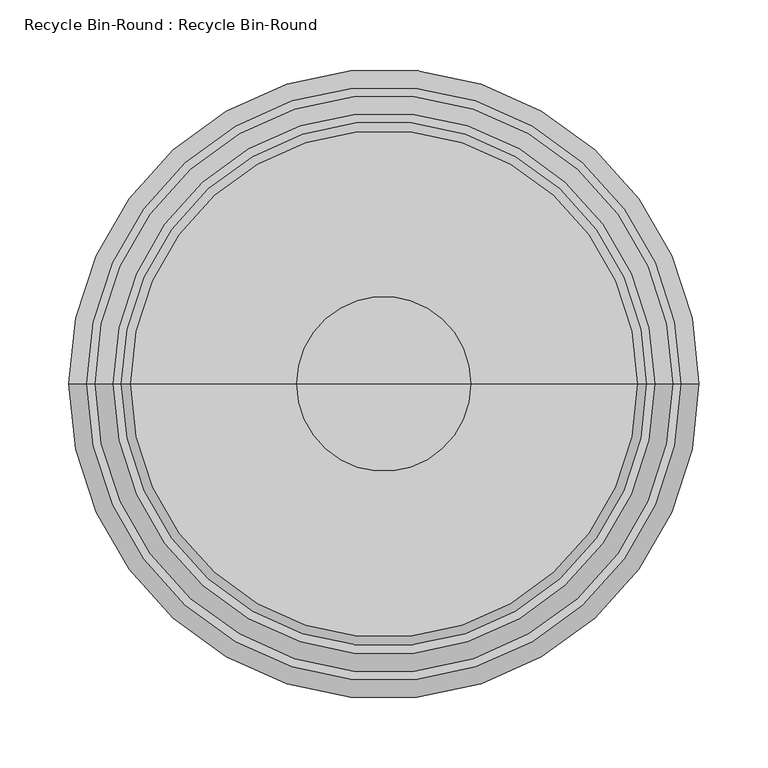
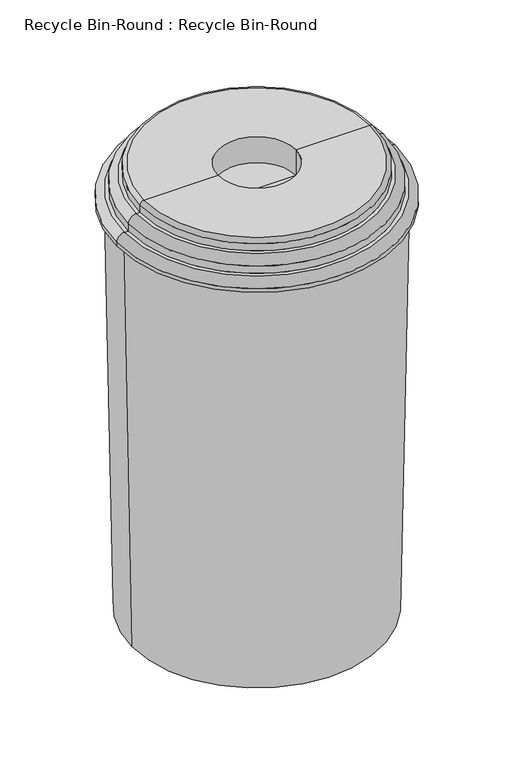
"""IFC4 building model written with IfcOpenShell, lengths in millimetres: proxy geometry, Recycle Bin-Round : Recycle Bin-Round."""

from ifc_helpers import new_model, si_unit, point, frame, origin, place, context, project, spatial, polyline, circle_curve, ellipse_curve, trimmed, source, transform, mapped, element, save
from ifc_brep_helpers import plane_surface, cylinder_surface, revolved_surface, advanced_brep


def recycle_bin_round_recycle_bin_round_6e7ed866(model_context):
    return source(origin(), model_context, "Body", "AdvancedBrep", [
        advanced_brep(
        [(-215.9, 0.0, 698.5), (215.9, 0.0, 698.5), (-203.2, 0.0, 0.0), (203.2, 0.0, 0.0)],
        [
            (0, 1, circle_curve(frame((0.0, 0.0, 698.5), z_axis=(0.0, 0.0, 1.0), x_axis=(-1.0, 0.0, 0.0)), 215.9)),
            (1, 0, circle_curve(frame((0.0, 0.0, 698.5), z_axis=(0.0, 0.0, 1.0), x_axis=(1.0, 0.0, 0.0)), 215.9)),
            (2, 3, circle_curve(frame((0.0, 0.0, 0.0), z_axis=(0.0, 0.0, -1.0), x_axis=(1.0, 0.0, 0.0)), 203.2)),
            (3, 2, circle_curve(frame((0.0, 0.0, 0.0), z_axis=(0.0, 0.0, -1.0), x_axis=(-1.0, 0.0, 0.0)), 203.2)),
            (3, 1),
            (0, 2),
        ],
        [
            plane_surface(frame((0.0, 0.0, 698.5), z_axis=(0.0, 0.0, 1.0), x_axis=(0.0, -1.0, 0.0))),
            plane_surface(frame((0.0, 0.0, 0.0), z_axis=(0.0, 0.0, -1.0), x_axis=(0.0, -1.0, 0.0))),
            revolved_surface(polyline([(203.2, 0.0, 0.0), (215.9, 0.0, 698.5)]), (0.0, 0.0, -11176.0), (0.0, 0.0, 1.0)),
            revolved_surface(polyline([(-203.2, 0.0, 0.0), (-215.9, 0.0, 698.5)]), (0.0, 0.0, -11176.0), (0.0, 0.0, 1.0)),
        ],
        [
            (0, [[1, 2]]),
            (1, [[3, 4]]),
            (2, [[-4, 5, -1, 6]]),
            (3, [[-3, -6, -2, -5]]),
        ],
    ),
        advanced_brep(
        [(-228.6, 0.0, 704.85), (228.6, 0.0, 704.85), (228.6, 0.0, 698.5), (-228.6, 0.0, 698.5), (-215.9, 0.0, 717.55), (215.9, 0.0, 717.55), (-209.55, 0.0, 717.55), (209.55, 0.0, 717.55), (-209.55, 0.0, 730.25), (209.55, 0.0, 730.25), (-196.85, 0.0, 742.95), (196.85, 0.0, 742.95), (-190.5, 0.0, 742.95), (190.5, 0.0, 742.95), (-190.5, 0.0, 755.65), (190.5, 0.0, 755.65), (-184.15, 0.0, 762.0), (184.15, 0.0, 762.0), (-63.5, 0.0, 762.0), (63.5, 0.0, 762.0), (-63.5, 0.0, 717.55), (63.5, 0.0, 717.55), (0.0, 0.0, 717.55), (0.0, 0.0, 698.5)],
        [
            (0, 1, circle_curve(frame((0.0, 0.0, 704.85), z_axis=(0.0, 0.0, -1.0), x_axis=(1.0, 0.0, 0.0)), 228.6)),
            (1, 2),
            (2, 3, circle_curve(frame((0.0, 0.0, 698.5), z_axis=(0.0, 0.0, 1.0), x_axis=(1.0, 0.0, 0.0)), 228.6)),
            (3, 0),
            (1, 0, circle_curve(frame((0.0, 0.0, 704.85), z_axis=(0.0, 0.0, -1.0), x_axis=(1.0, 0.0, 0.0)), 228.6)),
            (3, 2, circle_curve(frame((0.0, 0.0, 698.5), z_axis=(0.0, 0.0, 1.0), x_axis=(1.0, 0.0, 0.0)), 228.6)),
            (4, 5, circle_curve(frame((0.0, 0.0, 717.55), z_axis=(0.0, 0.0, -1.0), x_axis=(1.0, 0.0, 0.0)), 215.9)),
            (5, 1, circle_curve(frame((215.9, 0.0, 704.85), z_axis=(0.0, 1.0, 0.0), x_axis=(1.0, 0.0, 0.0)), 12.7)),
            (0, 4, circle_curve(frame((-215.9, 0.0, 704.85), z_axis=(0.0, 1.0, 0.0), x_axis=(-1.0, 0.0, 0.0)), 12.7)),
            (5, 4, circle_curve(frame((0.0, 0.0, 717.55), z_axis=(0.0, 0.0, -1.0), x_axis=(1.0, 0.0, 0.0)), 215.9)),
            (6, 7, circle_curve(frame((0.0, 0.0, 717.55), z_axis=(0.0, 0.0, -1.0), x_axis=(1.0, 0.0, 0.0)), 209.55)),
            (7, 5),
            (4, 6),
            (7, 6, circle_curve(frame((0.0, 0.0, 717.55), z_axis=(0.0, 0.0, -1.0), x_axis=(1.0, 0.0, 0.0)), 209.55)),
            (8, 9, circle_curve(frame((0.0, 0.0, 730.25), z_axis=(0.0, 0.0, -1.0), x_axis=(1.0, 0.0, 0.0)), 209.55)),
            (9, 7),
            (6, 8),
            (9, 8, circle_curve(frame((0.0, 0.0, 730.25), z_axis=(0.0, 0.0, -1.0), x_axis=(1.0, 0.0, 0.0)), 209.55)),
            (10, 11, circle_curve(frame((0.0, 0.0, 742.95), z_axis=(0.0, 0.0, -1.0), x_axis=(1.0, 0.0, 0.0)), 196.85)),
            (11, 9, circle_curve(frame((196.85, 0.0, 730.25), z_axis=(0.0, 1.0, 0.0), x_axis=(1.0, 0.0, 0.0)), 12.7)),
            (8, 10, circle_curve(frame((-196.85, 0.0, 730.25), z_axis=(0.0, 1.0, 0.0), x_axis=(-1.0, 0.0, 0.0)), 12.7)),
            (11, 10, circle_curve(frame((0.0, 0.0, 742.95), z_axis=(0.0, 0.0, -1.0), x_axis=(1.0, 0.0, 0.0)), 196.85)),
            (12, 13, circle_curve(frame((0.0, 0.0, 742.95), z_axis=(0.0, 0.0, -1.0), x_axis=(1.0, 0.0, 0.0)), 190.5)),
            (13, 11),
            (10, 12),
            (13, 12, circle_curve(frame((0.0, 0.0, 742.95), z_axis=(0.0, 0.0, -1.0), x_axis=(1.0, 0.0, 0.0)), 190.5)),
            (14, 15, circle_curve(frame((0.0, 0.0, 755.65), z_axis=(0.0, 0.0, -1.0), x_axis=(1.0, 0.0, 0.0)), 190.5)),
            (15, 13),
            (12, 14),
            (15, 14, circle_curve(frame((0.0, 0.0, 755.65), z_axis=(0.0, 0.0, -1.0), x_axis=(1.0, 0.0, 0.0)), 190.5)),
            (16, 17, circle_curve(frame((0.0, 0.0, 762.0), z_axis=(0.0, 0.0, -1.0), x_axis=(1.0, 0.0, 0.0)), 184.15)),
            (17, 15, circle_curve(frame((184.15, 0.0, 755.65), z_axis=(0.0, 1.0, 0.0), x_axis=(1.0, 0.0, 0.0)), 6.35)),
            (14, 16, circle_curve(frame((-184.15, 0.0, 755.65), z_axis=(0.0, 1.0, 0.0), x_axis=(-1.0, 0.0, 0.0)), 6.35)),
            (17, 16, circle_curve(frame((0.0, 0.0, 762.0), z_axis=(0.0, 0.0, -1.0), x_axis=(1.0, 0.0, 0.0)), 184.15)),
            (18, 19, circle_curve(frame((0.0, 0.0, 762.0), z_axis=(0.0, 0.0, -1.0), x_axis=(1.0, 0.0, 0.0)), 63.5)),
            (19, 17),
            (16, 18),
            (19, 18, circle_curve(frame((0.0, 0.0, 762.0), z_axis=(0.0, 0.0, -1.0), x_axis=(1.0, 0.0, 0.0)), 63.5)),
            (20, 21, circle_curve(frame((0.0, 0.0, 717.55), z_axis=(0.0, 0.0, -1.0), x_axis=(1.0, 0.0, 0.0)), 63.5)),
            (21, 19),
            (18, 20),
            (21, 20, circle_curve(frame((0.0, 0.0, 717.55), z_axis=(0.0, 0.0, -1.0), x_axis=(1.0, 0.0, 0.0)), 63.5)),
            (22, 21),
            (20, 22),
            (2, 23),
            (23, 3),
        ],
        [
            cylinder_surface(frame((0.0, 0.0, 698.5), z_axis=(0.0, 0.0, 1.0), x_axis=(1.0, 0.0, 0.0)), 228.6),
            revolved_surface(trimmed(ellipse_curve(frame((215.9, 0.0, 704.85), z_axis=(0.0, -1.0, 0.0), x_axis=(1.0, 0.0, 0.0)), 12.7, 12.7), [point((228.6, 0.0, 704.85))], [point((215.9, 0.0, 717.55))], True, "CARTESIAN"), (0.0, 0.0, 698.5), (0.0, 0.0, 1.0)),
            plane_surface(frame((0.0, 0.0, 717.55), z_axis=(0.0, 0.0, 1.0), x_axis=(1.0, 0.0, 0.0))),
            cylinder_surface(frame((0.0, 0.0, 698.5), z_axis=(0.0, 0.0, 1.0), x_axis=(1.0, 0.0, 0.0)), 209.55),
            revolved_surface(trimmed(ellipse_curve(frame((196.85, 0.0, 730.25), z_axis=(0.0, -1.0, 0.0), x_axis=(1.0, 0.0, 0.0)), 12.7, 12.7), [point((209.55, 0.0, 730.25))], [point((196.85, 0.0, 742.95))], True, "CARTESIAN"), (0.0, 0.0, 698.5), (0.0, 0.0, 1.0)),
            plane_surface(frame((0.0, 0.0, 742.95), z_axis=(0.0, 0.0, 1.0), x_axis=(1.0, 0.0, 0.0))),
            cylinder_surface(frame((0.0, 0.0, 698.5), z_axis=(0.0, 0.0, 1.0), x_axis=(1.0, 0.0, 0.0)), 190.5),
            revolved_surface(trimmed(ellipse_curve(frame((184.15, 0.0, 755.65), z_axis=(0.0, -1.0, 0.0), x_axis=(1.0, 0.0, 0.0)), 6.35, 6.35), [point((190.5, 0.0, 755.65))], [point((184.15, 0.0, 762.0))], True, "CARTESIAN"), (0.0, 0.0, 698.5), (0.0, 0.0, 1.0)),
            plane_surface(frame((0.0, 0.0, 762.0), z_axis=(0.0, 0.0, 1.0), x_axis=(1.0, 0.0, 0.0))),
            revolved_surface(polyline([(63.5, 0.0, 762.0), (63.5, 0.0, 717.55)]), (0.0, 0.0, 698.5), (0.0, 0.0, 1.0)),
            plane_surface(frame((0.0, 0.0, 698.5), z_axis=(0.0, 0.0, -1.0), x_axis=(1.0, 0.0, 0.0))),
        ],
        [
            (0, [[1, 2, 3, 4]]),
            (0, [[5, -4, 6, -2]]),
            (1, [[7, 8, -1, 9]]),
            (1, [[10, -9, -5, -8]]),
            (2, [[11, 12, -7, 13]]),
            (2, [[14, -13, -10, -12]]),
            (3, [[15, 16, -11, 17]]),
            (3, [[18, -17, -14, -16]]),
            (4, [[19, 20, -15, 21]]),
            (4, [[22, -21, -18, -20]]),
            (5, [[23, 24, -19, 25]]),
            (5, [[26, -25, -22, -24]]),
            (6, [[27, 28, -23, 29]]),
            (6, [[30, -29, -26, -28]]),
            (7, [[31, 32, -27, 33]]),
            (7, [[34, -33, -30, -32]]),
            (8, [[35, 36, -31, 37]]),
            (8, [[38, -37, -34, -36]]),
            (9, [[39, 40, -35, 41]]),
            (9, [[42, -41, -38, -40]]),
            (2, [[43, -39, 44]]),
            (2, [[-44, -42, -43]]),
            (10, [[-3, 45, 46]]),
            (10, [[-6, -46, -45]]),
        ],
    ),
    ])


if __name__ == "__main__":
    model = new_model("IFC4")
    model_context = context("Model", 3, world=origin())
    ifc_project = project(units=[si_unit("LENGTHUNIT", "METRE", prefix="MILLI")], contexts=[model_context])
    site = spatial("IfcSite", under=ifc_project)
    building = spatial("IfcBuilding", under=site)
    placement = place(None, origin())
    recycle_bin_round_recycle_bin_round_shape = recycle_bin_round_recycle_bin_round_6e7ed866(model_context)
    element("IfcBuildingElementProxy", 1, Name="Recycle Bin-Round : Recycle Bin-Round", ObjectType="Recycle Bin-Round : Recycle Bin-Round", at=placement, inside=building, context=model_context, shape_type="MappedRepresentation", body=[
        mapped(recycle_bin_round_recycle_bin_round_shape, transform((0.0, 0.0, 0.0), x_axis=(1.0, 0.0, 0.0), y_axis=(0.0, 1.0, 0.0), z_axis=(0.0, 0.0, 1.0))),
    ])
    save(model, "model.ifc")

# Revit data of these elements
# Type "Recycle Bin-Round : Recycle Bin-Round"
#   Default Elevation = 0
# Element 1 (IfcBuildingElementProxy, "Recycle Bin-Round : Recycle Bin-Round")
#   Materials on its faces: "Plastic - Blue", "Default - Black"
# Materials
#   "Plastic - Blue": class "Plastic", colour RGB 0 0 212, transparency 0
#   "Default - Black": colour RGB 0 0 0, transparency 0
